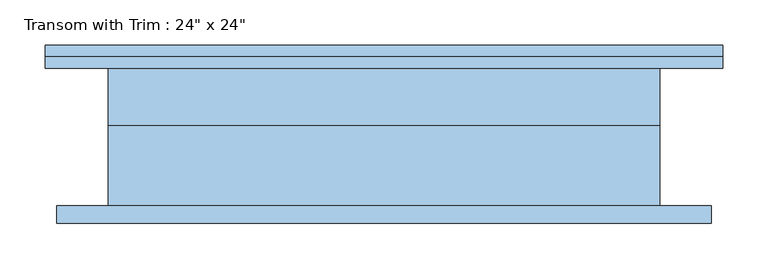
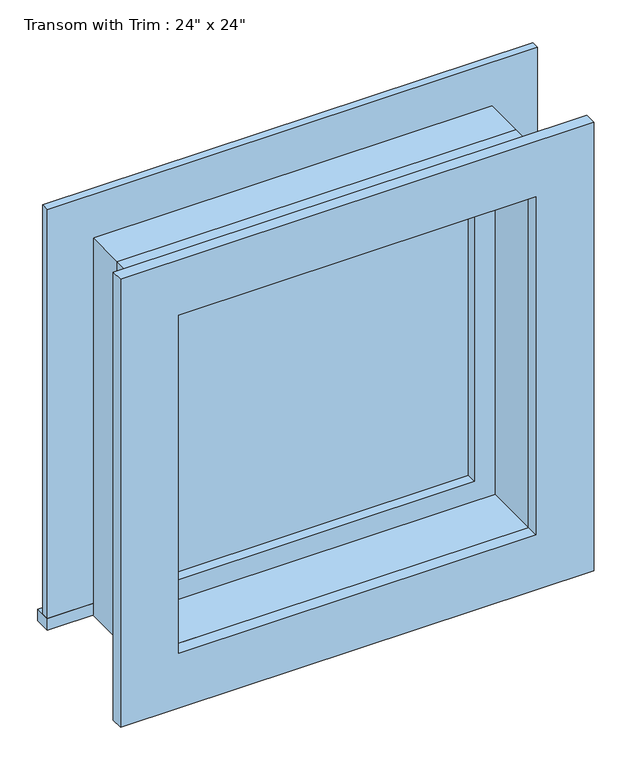
"""IFC4 building model written with IfcOpenShell, lengths in millimetres: window geometry."""

from ifc_helpers import new_model, si_unit, frame, origin, place, context, project, spatial, polyline, outline, extrude, source, transform, mapped, element, save


def window_3d781103(model_context):
    return source(origin(), model_context, "Body", "SweptSolid", [
        extrude(outline(polyline([(-412.75, 101.6), (336.55, 101.6), (336.55, 76.2), (-412.75, 76.2), (-412.75, 101.6)])), frame((0.0, 0.0, 2159.0), z_axis=(0.0, 0.0, 1.0), x_axis=(1.0, 0.0, 0.0)), (0.0, 0.0, 1.0), 19.05),
        extrude(outline(polyline([(2749.55, -323.85), (2749.55, 247.65), (2178.05, 247.65), (2178.05, 336.55), (2838.45, 336.55), (2838.45, -412.75), (2178.05, -412.75), (2178.05, -323.85), (2749.55, -323.85)])), frame((0.0, 76.2, 0.0), z_axis=(0.0, 1.0, 0.0), x_axis=(0.0, 0.0, 1.0)), (0.0, 0.0, 1.0), 12.7),
        extrude(outline(polyline([(2825.75, 323.85), (2825.75, -400.05), (2101.85, -400.05), (2101.85, 323.85), (2825.75, 323.85)]), holes=[polyline([(2736.85, 234.95), (2190.75, 234.95), (2190.75, -311.15), (2736.85, -311.15), (2736.85, 234.95)])]), frame((0.0, -95.25, 0.0), z_axis=(0.0, 1.0, 0.0), x_axis=(0.0, 0.0, 1.0)), (0.0, 0.0, 1.0), 19.05),
        extrude(outline(polyline([(203.2, 28.575), (-279.4, 28.575), (-279.4, 41.275), (203.2, 41.275), (203.2, 28.575)])), frame((0.0, 0.0, 2222.5), z_axis=(0.0, 0.0, 1.0), x_axis=(1.0, 0.0, 0.0)), (0.0, 0.0, 1.0), 482.6),
        extrude(outline(polyline([(2749.55, -323.85), (2178.05, -323.85), (2178.05, 247.65), (2749.55, 247.65), (2749.55, -323.85)]), holes=[polyline([(2705.1, -279.4), (2705.1, 203.2), (2222.5, 203.2), (2222.5, -279.4), (2705.1, -279.4)])]), frame((0.0, 12.7, 0.0), z_axis=(0.0, 1.0, 0.0), x_axis=(0.0, 0.0, 1.0)), (0.0, 0.0, 1.0), 44.45),
        extrude(outline(polyline([(2768.6, -342.9), (2159.0, -342.9), (2159.0, 266.7), (2768.6, 266.7), (2768.6, -342.9)]), holes=[polyline([(2736.85, -311.15), (2736.85, 234.95), (2190.75, 234.95), (2190.75, -311.15), (2736.85, -311.15)])]), frame((0.0, -76.2, 0.0), z_axis=(0.0, 1.0, 0.0), x_axis=(0.0, 0.0, 1.0)), (0.0, 0.0, 1.0), 88.9),
        extrude(outline(polyline([(2768.6, 266.7), (2768.6, -342.9), (2159.0, -342.9), (2159.0, 266.7), (2768.6, 266.7)]), holes=[polyline([(2749.55, 247.65), (2178.05, 247.65), (2178.05, -323.85), (2749.55, -323.85), (2749.55, 247.65)])]), frame((0.0, 12.7, 0.0), z_axis=(0.0, 1.0, 0.0), x_axis=(0.0, 0.0, 1.0)), (0.0, 0.0, 1.0), 63.5),
    ])


if __name__ == "__main__":
    model = new_model("IFC4")
    model_context = context("Model", 3, world=origin())
    ifc_project = project(units=[si_unit("LENGTHUNIT", "METRE", prefix="MILLI")], contexts=[model_context])
    site = spatial("IfcSite", under=ifc_project)
    building = spatial("IfcBuilding", under=site)
    placement = place(None, origin())
    window_shape = window_3d781103(model_context)
    element("IfcWindow", 1, ObjectType="Transom with Trim : 24\" x 24\"", at=placement, inside=building, context=model_context, shape_type="MappedRepresentation", body=[
        mapped(window_shape, transform((0.0, 0.0, 0.0), x_axis=(1.0, 0.0, 0.0), y_axis=(0.0, 1.0, 0.0), z_axis=(0.0, 0.0, 1.0))),
    ])
    save(model, "model.ifc")

# Revit data of these elements
# Type "Transom with Trim : 24\" x 24\""
#   Type Mark = "10"
#   Construction Type Id = "GSP4R"
#   Assembly Code = "B2020100"
#   Analytic Construction = "1/8 in Pilkington single glazing"
#   Visual Light Transmittance = 0.9
#   Solar Heat Gain Coefficient = 0.78
#   Heat Transfer Coefficient (U) = 0.6496 BTU/(h·ft²·°F)
#   Height = 2' - 0"
#   Default Sill Height = 7' - 1"
#   Trim Projection - Ext. = 0' - 0 1/2"
#   Trim Projection - Int. = 0' - 0 3/4"
#   Trim Width - Exterior = 0' - 3 1/2"
#   Trim Width - Interior = 0' - 3 1/2"
#   Width = 2' - 0"
#   Window Inset = 0' - 0 3/4"
#   Define Thermal Properties by = 1
#   Glass Pane Material = Glass
#   Sash Material = Sash
#   Trim Exterior Material = Trim
#   Trim Interior Material = Trim
#   Wall Closure = (empty or 0)
# Element 1 (IfcWindow, "Transom with Trim : 24\" x 24\"")
#   Materials on its faces: "Sash", "Trim", "Glass"
# Materials
#   "Glass": class "Glass", colour RGB 0 128 192, transparency 0.75, Description = "Soda Lime Glass", Cost = 0
#   "Sash": class "Wood", colour RGB 224 178 126, transparency 0
#   "Trim": class "Wood", colour RGB 224 178 126, transparency 0
